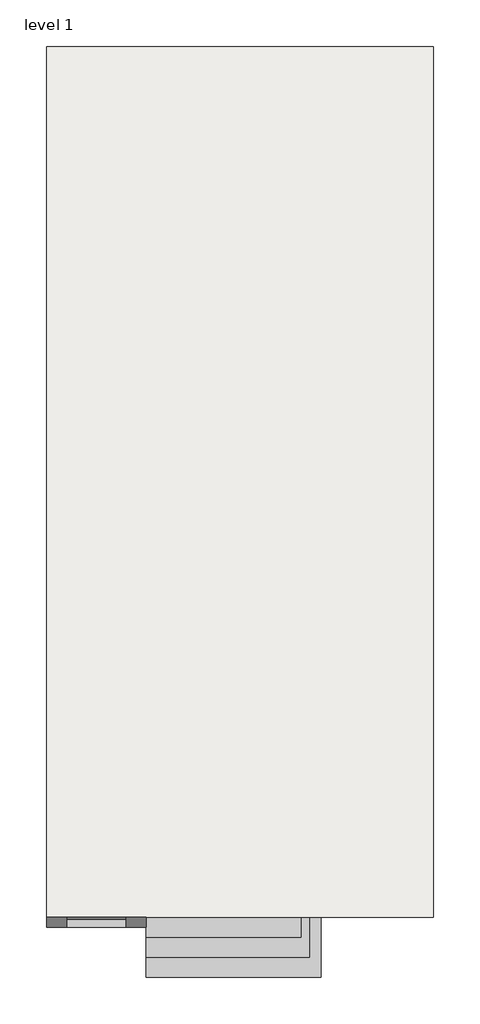
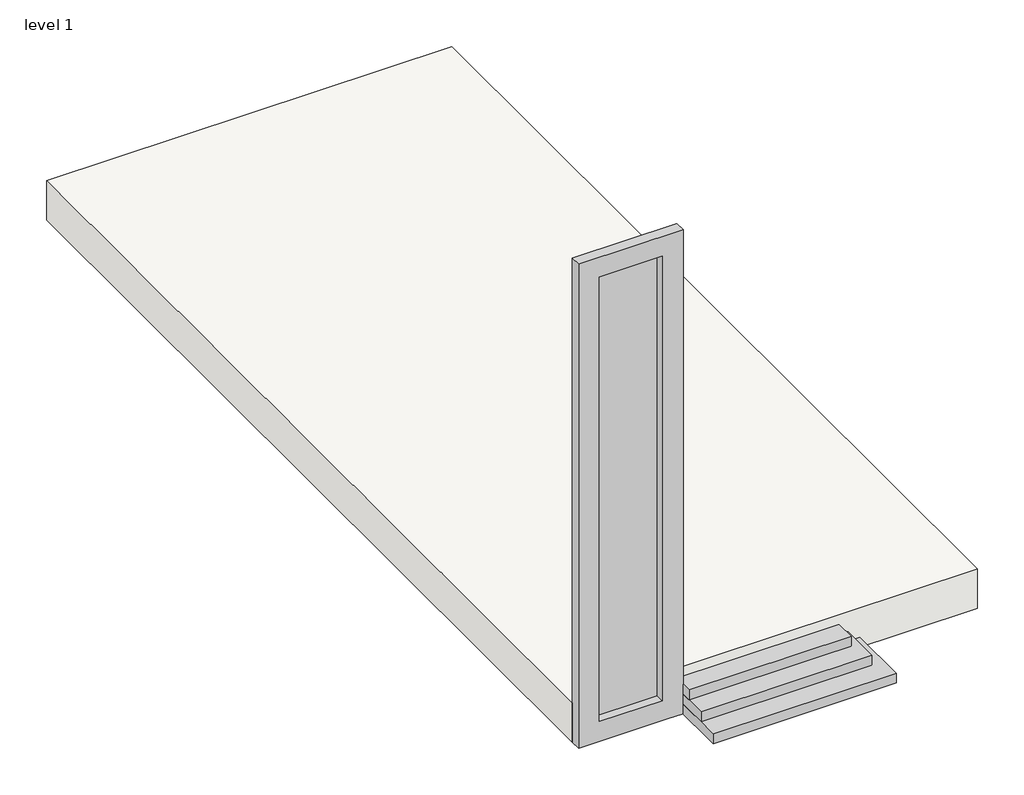
# One storey: 4 proxies, 1 slab.
"""IFC4 building model written with IfcOpenShell, lengths in millimetres."""

from ifc_helpers import new_model, si_unit, origin, origin_with_axes, place, context, project, spatial, polyline, outline, extrude, transform, mapped, element, save
from components import generic_models_15_generic_models_15_a6985b4b, generic_models_2_generic_models_2_72429bd6, generic_models_3_generic_models_3_af6268f2, generic_models_4_generic_models_4_a39c55b3

model = new_model("IFC4")

# Units and contexts
model_context = context("Model", 3, world=origin())
ifc_project = project(units=[si_unit("LENGTHUNIT", "METRE", prefix="MILLI")], contexts=[model_context])

# Site, building, storey
site = spatial("IfcSite", under=ifc_project)
building = spatial("IfcBuilding", under=site)
storey = spatial("IfcBuildingStorey", under=building, Name="level 1", Elevation=0.0)

# Proxies
placement = place(None, origin())
generic_models_15_generic_models_15_shape = generic_models_15_generic_models_15_a6985b4b(model_context)
element("IfcBuildingElementProxy", 1, Name="Generic Models 15 : Generic Models 15", ObjectType="Generic Models 15 : Generic Models 15", at=placement, inside=storey, context=model_context, shape_type="MappedRepresentation", body=[
    mapped(generic_models_15_generic_models_15_shape, transform((0.0, 0.0, 0.0), x_axis=(1.0, 0.0, 0.0), y_axis=(0.0, 1.0, 0.0), z_axis=(0.0, 0.0, 1.0))),
])
generic_models_2_generic_models_2_shape = generic_models_2_generic_models_2_72429bd6(model_context)
element("IfcBuildingElementProxy", 2, Name="Generic Models 2 : Generic Models 2", ObjectType="Generic Models 2 : Generic Models 2", at=placement, inside=storey, context=model_context, shape_type="MappedRepresentation", body=[
    mapped(generic_models_2_generic_models_2_shape, transform((0.0, 0.0, 0.0), x_axis=(1.0, 0.0, 0.0), y_axis=(0.0, 1.0, 0.0), z_axis=(0.0, 0.0, 1.0))),
])
generic_models_3_generic_models_3_shape = generic_models_3_generic_models_3_af6268f2(model_context)
element("IfcBuildingElementProxy", 3, Name="Generic Models 3 : Generic Models 3", ObjectType="Generic Models 3 : Generic Models 3", at=placement, inside=storey, context=model_context, shape_type="MappedRepresentation", body=[
    mapped(generic_models_3_generic_models_3_shape, transform((0.0, 0.0, 0.0), x_axis=(1.0, 0.0, 0.0), y_axis=(0.0, 1.0, 0.0), z_axis=(0.0, 0.0, 1.0))),
])
generic_models_4_generic_models_4_shape = generic_models_4_generic_models_4_a39c55b3(model_context)
element("IfcBuildingElementProxy", 4, Name="Generic Models 4 : Generic Models 4", ObjectType="Generic Models 4 : Generic Models 4", at=placement, inside=storey, context=model_context, shape_type="MappedRepresentation", body=[
    mapped(generic_models_4_generic_models_4_shape, transform((0.0, 0.0, 0.0), x_axis=(1.0, 0.0, 0.0), y_axis=(0.0, 1.0, 0.0), z_axis=(0.0, 0.0, 1.0))),
])

# Slab
element("IfcSlab", 5, ObjectType="floor 2'", at=placement, inside=storey, context=model_context, shape_type="SweptSolid", body=[
    extrude(outline(polyline([(-10521.0371373, 9903.938593), (-10521.0371373, -3380.261407), (-16426.5371373, -3380.261407), (-16426.5371373, 9903.938593), (-10521.0371373, 9903.938593)])), origin_with_axes(), (0.0, 0.0, 1.0), 609.6),
])

save(model, "model.ifc")

# Revit data of these elements
# Type "floor 2'"
#   Assembly Code = "B1010"
#   Function = 0
#   Layers, outside or top first: 2' - 0" no material (function 1)
# Element 1 (IfcBuildingElementProxy, "Generic Models 15 : Generic Models 15")
#   Phase Created = New Construction
#   Materials on its faces: "2.FRONT WALL PAINT"
# Element 2 (IfcBuildingElementProxy, "Generic Models 2 : Generic Models 2")
#   Phase Created = New Construction
# Element 3 (IfcBuildingElementProxy, "Generic Models 3 : Generic Models 3")
#   Phase Created = New Construction
# Element 4 (IfcBuildingElementProxy, "Generic Models 4 : Generic Models 4")
#   Phase Created = New Construction
# Element 5 (IfcSlab, "floor 2'")
#   Height Offset From Level = 2' - 0"
#   Phase Created = New Construction
#   Materials on its faces: "5. GRAVEL"
# Materials
#   "2.FRONT WALL PAINT": class "Generic", colour RGB 120 120 120, transparency 0, Cost = 0
#   "5. GRAVEL": class "Generic", colour RGB 120 120 120, transparency 0, Cost = 0
